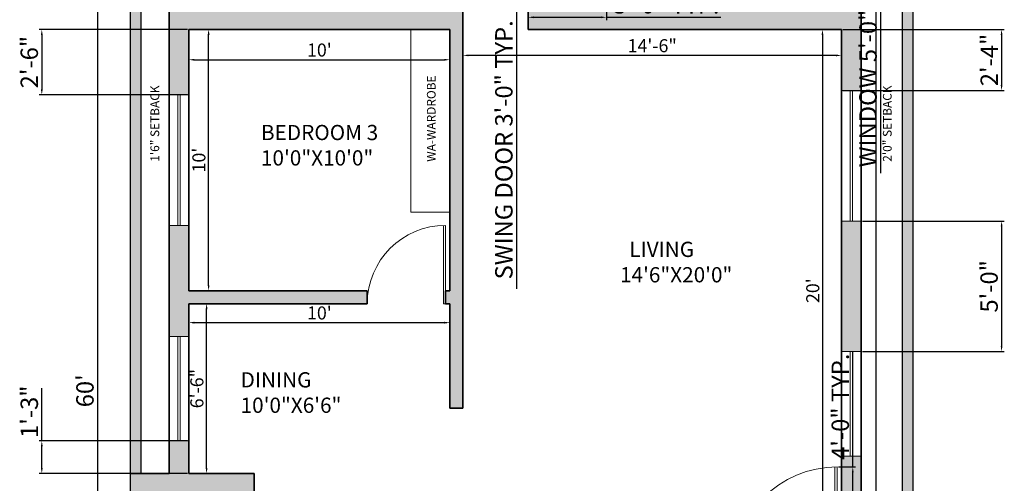
# Model space of a CAD drawing. Units: inches. Extents: x 2700 to 4052, y 1030 to 1872.
# Tile 7 of 8: x 3518 to 3971, y 1419 to 1632. Entities that reach past the tile are written whole.
import ezdxf

# ---------------------------------------------------------------- set-up
doc = ezdxf.new("R2010")
doc.units = ezdxf.units.IN
for name, color, linetype, lineweight in [('A-ANNO-DIMS', 2, 'Continuous', 13), ('A-ANNO-TEXT', 7, 'Continuous', 18), ('A-AREA-IDEN', 7, 'Continuous', 18), ('A-DOOR', 4, 'Continuous', 18), ('A-FLOR-CASE', 8, 'Continuous', 18), ('A-GLAZ', 4, 'Continuous', 18), ('A-WALL', 7, 'Continuous', 35), ('A-WALL-PATT', 7, 'Continuous', 13), ('C-PROP', 7, 'Continuous', 25)]:
    doc.layers.add(name, color=color, linetype=linetype, lineweight=lineweight)
doc.layers.add('C-SITE-PATT', color=252, linetype='Continuous', lineweight=13, true_color=0x939598)
doc.styles.get("Standard").update_dxf_attribs({"font": 'arial.ttf'})
doc.dimstyles.new('ISO-25', dxfattribs={"dimtxt": 8, "dimasz": 2.5, "dimexe": 1.25, "dimexo": 0.625, "dimtad": 1, "dimdec": 1, "dimlunit": 3, "dimtxsty": 'Standard', "dimcen": 2.5, "dimclrt": 1, "dimadec": 0, "dimazin": 0, "dimtfac": 1, "dimtdec": 1, "dimtmove": 0, "dimatfit": 3, "dimfxl": 1, "dimarcsym": 0})

# ---------------------------------------------------------------- blocks, each defined once
blk = doc.blocks.new('*D22')
at = {"layer": 'A-ANNO-DIMS', "color": 0, "lineweight": -2, "transparency": 16777216}
for p, q in [((3568.26, 1821.52), (3552.61, 1821.52)), ((3553.86, 1819.02), (3553.86, 1104.02)), ((3568.26, 1101.52), (3552.61, 1101.52))]:
    blk.add_line(p, q, dxfattribs=at)
at = {"layer": 'A-ANNO-DIMS', "color": 0, "transparency": 16777216}
for points in [[(3553.44, 1819.02), (3554.28, 1819.02), (3553.86, 1821.52)], [(3553.44, 1104.02), (3554.28, 1104.02), (3553.86, 1101.52)]]:
    blk.add_solid(points, dxfattribs=at)
at = {"layer": 'Defpoints', "color": 0, "transparency": 16777216}
for p in [(3568.88, 1821.52), (3553.86, 1101.52), (3568.88, 1101.52)]:
    blk.add_point(p, dxfattribs=at)
at = {"layer": 'A-ANNO-DIMS', "color": 0, "transparency": 16777216, "insert": (3549.15, 1461.52), "char_height": 8, "attachment_point": 5, "rotation": 90}
blk.add_mtext("60'", dxfattribs=at)
blk = doc.blocks.new('*D36')
at = {"layer": 'A-ANNO-DIMS', "color": 0, "lineweight": -2, "transparency": 16777216}
for p, q in [((3596.51, 1501.52), (3605.29, 1501.52)), ((3604.04, 1426.02), (3604.04, 1499.02)), ((3596.51, 1423.52), (3605.29, 1423.52))]:
    blk.add_line(p, q, dxfattribs=at)
at = {"layer": 'A-ANNO-DIMS', "color": 0, "transparency": 16777216}
for points in [[(3603.62, 1499.02), (3604.45, 1499.02), (3604.04, 1501.52)], [(3603.62, 1426.02), (3604.45, 1426.02), (3604.04, 1423.52)]]:
    blk.add_solid(points, dxfattribs=at)
at = {"layer": 'Defpoints', "color": 0, "transparency": 16777216}
for p in [(3595.88, 1501.52), (3604.04, 1501.52), (3595.88, 1423.52)]:
    blk.add_point(p, dxfattribs=at)
at = {"layer": 'A-ANNO-DIMS', "color": 0, "transparency": 16777216, "insert": (3600.35, 1462.52), "char_height": 6, "attachment_point": 5, "rotation": 90}
blk.add_mtext('6\'-6"', dxfattribs=at)
blk = doc.blocks.new('*D37')
at = {"layer": 'A-ANNO-DIMS', "color": 0, "lineweight": -2, "transparency": 16777216}
for p, q in [((3595.88, 1500.89), (3595.88, 1491.57)), ((3715.88, 1500.89), (3715.88, 1491.57)), ((3598.38, 1492.82), (3713.38, 1492.82))]:
    blk.add_line(p, q, dxfattribs=at)
at = {"layer": 'A-ANNO-DIMS', "color": 0, "transparency": 16777216}
for points in [[(3598.38, 1493.24), (3598.38, 1492.4), (3595.88, 1492.82)], [(3713.38, 1493.24), (3713.38, 1492.4), (3715.88, 1492.82)]]:
    blk.add_solid(points, dxfattribs=at)
at = {"layer": 'Defpoints', "color": 0, "transparency": 16777216}
for p in [(3595.88, 1501.52), (3715.88, 1501.52), (3715.88, 1492.82)]:
    blk.add_point(p, dxfattribs=at)
at = {"layer": 'A-ANNO-DIMS', "color": 0, "transparency": 16777216, "insert": (3655.88, 1496.51), "char_height": 6, "attachment_point": 5}
blk.add_mtext("10'", dxfattribs=at)
blk = doc.blocks.new('*D38')
at = {"layer": 'A-ANNO-DIMS', "color": 0, "lineweight": -2, "transparency": 16777216}
for p, q in [((3596.51, 1627.52), (3606.21, 1627.52)), ((3604.96, 1510.02), (3604.96, 1625.02)), ((3596.51, 1507.52), (3606.21, 1507.52))]:
    blk.add_line(p, q, dxfattribs=at)
at = {"layer": 'A-ANNO-DIMS', "color": 0, "transparency": 16777216}
for points in [[(3604.54, 1625.02), (3605.38, 1625.02), (3604.96, 1627.52)], [(3604.54, 1510.02), (3605.38, 1510.02), (3604.96, 1507.52)]]:
    blk.add_solid(points, dxfattribs=at)
at = {"layer": 'Defpoints', "color": 0, "transparency": 16777216}
for p in [(3595.88, 1627.52), (3604.96, 1627.52), (3595.88, 1507.52)]:
    blk.add_point(p, dxfattribs=at)
at = {"layer": 'A-ANNO-DIMS', "color": 0, "transparency": 16777216, "insert": (3601.27, 1567.52), "char_height": 6, "attachment_point": 5, "rotation": 90}
blk.add_mtext("10'", dxfattribs=at)
blk = doc.blocks.new('*D39')
at = {"layer": 'A-ANNO-DIMS', "color": 0, "lineweight": -2, "transparency": 16777216}
for p, q in [((3595.88, 1626.89), (3595.88, 1612.37)), ((3715.88, 1626.89), (3715.88, 1612.37)), ((3598.38, 1613.62), (3713.38, 1613.62))]:
    blk.add_line(p, q, dxfattribs=at)
at = {"layer": 'A-ANNO-DIMS', "color": 0, "transparency": 16777216}
for points in [[(3598.38, 1614.04), (3598.38, 1613.2), (3595.88, 1613.62)], [(3713.38, 1614.04), (3713.38, 1613.2), (3715.88, 1613.62)]]:
    blk.add_solid(points, dxfattribs=at)
at = {"layer": 'Defpoints', "color": 0, "transparency": 16777216}
for p in [(3595.88, 1627.52), (3715.88, 1627.52), (3715.88, 1613.62)]:
    blk.add_point(p, dxfattribs=at)
at = {"layer": 'A-ANNO-DIMS', "color": 0, "transparency": 16777216, "insert": (3655.88, 1617.31), "char_height": 6, "attachment_point": 5}
blk.add_mtext("10'", dxfattribs=at)
blk = doc.blocks.new('*D47')
at = {"layer": 'A-ANNO-DIMS', "color": 0, "lineweight": -2, "transparency": 16777216}
for p, q in [((3721.88, 1626.89), (3721.88, 1614.36)), ((3895.88, 1626.89), (3895.88, 1614.36)), ((3893.38, 1615.61), (3724.38, 1615.61))]:
    blk.add_line(p, q, dxfattribs=at)
at = {"layer": 'A-ANNO-DIMS', "color": 0, "transparency": 16777216}
for points in [[(3724.38, 1616.03), (3724.38, 1615.2), (3721.88, 1615.61)], [(3893.38, 1616.03), (3893.38, 1615.2), (3895.88, 1615.61)]]:
    blk.add_solid(points, dxfattribs=at)
at = {"layer": 'Defpoints', "color": 0, "transparency": 16777216}
for p in [(3721.88, 1627.52), (3895.88, 1627.52), (3721.88, 1615.61)]:
    blk.add_point(p, dxfattribs=at)
at = {"layer": 'A-ANNO-DIMS', "color": 0, "transparency": 16777216, "insert": (3808.88, 1619.3), "char_height": 6, "attachment_point": 5}
blk.add_mtext('14\'-6"', dxfattribs=at)
blk = doc.blocks.new('*D49')
at = {"layer": 'A-ANNO-DIMS', "color": 0, "lineweight": -2, "transparency": 16777216}
for p, q in [((3895.26, 1627.52), (3885.9, 1627.52)), ((3887.15, 1625.02), (3887.15, 1390.02)), ((3895.26, 1387.52), (3885.9, 1387.52))]:
    blk.add_line(p, q, dxfattribs=at)
at = {"layer": 'A-ANNO-DIMS', "color": 0, "transparency": 16777216}
for points in [[(3886.73, 1625.02), (3887.57, 1625.02), (3887.15, 1627.52)], [(3886.73, 1390.02), (3887.57, 1390.02), (3887.15, 1387.52)]]:
    blk.add_solid(points, dxfattribs=at)
at = {"layer": 'Defpoints', "color": 0, "transparency": 16777216}
for p in [(3895.88, 1627.52), (3887.15, 1387.52), (3895.88, 1387.52)]:
    blk.add_point(p, dxfattribs=at)
at = {"layer": 'A-ANNO-DIMS', "color": 0, "transparency": 16777216, "insert": (3883.46, 1507.52), "char_height": 6, "attachment_point": 5, "rotation": 90}
blk.add_mtext("20'", dxfattribs=at)
blk = doc.blocks.new('DOOR-SWING-48IN')
for p, q in [((-1, 48), (-1, 0)), ((0, 48), (0, 0)), ((0, 0), (-1, 0))]:
    blk.add_line(p, q)
blk.add_arc((0, 0), 48, 90, 180)
blk = doc.blocks.new('DOOR-SWING-36IN')
for p, q in [((-1, 36), (-1, 0)), ((0, 36), (0, 0)), ((0, 0), (-1, 0))]:
    blk.add_line(p, q)
blk.add_arc((0, 0), 36, 90, 180)
blk = doc.blocks.new('WINDOW-48IN')
for p, q in [((-24, -4.5), (-24, 4.5)), ((-24, 0.5), (24, 0.5)), ((24, -4.5), (24, 4.5)), ((-24, -0.5), (24, -0.5))]:
    blk.add_line(p, q)
blk = doc.blocks.new('WINDOW-60IN')
for p, q in [((4.5, 30), (-4.5, 30)), ((-0.5, 30), (-0.5, -30)), ((0.5, 30), (0.5, -30)), ((4.5, -30), (-4.5, -30))]:
    blk.add_line(p, q)
blk = doc.blocks.new('*D66')
at = {"layer": 'A-ANNO-DIMS', "color": 0, "lineweight": -2, "transparency": 16777216}
for p, q in [((3905.51, 1726.52), (3915.13, 1726.52)), ((3913.88, 1724.02), (3913.88, 1669.02)), ((3905.51, 1666.52), (3915.13, 1666.52)), ((3913.88, 1666.52), (3913.88, 1561.53))]:
    blk.add_line(p, q, dxfattribs=at)
at = {"layer": 'A-ANNO-DIMS', "color": 0, "transparency": 16777216}
for points in [[(3913.47, 1724.02), (3914.3, 1724.02), (3913.88, 1726.52)], [(3913.47, 1669.02), (3914.3, 1669.02), (3913.88, 1666.52)]]:
    blk.add_solid(points, dxfattribs=at)
at = {"layer": 'Defpoints', "color": 0, "transparency": 16777216}
for p in [(3904.88, 1726.52), (3904.88, 1666.52), (3913.88, 1666.52)]:
    blk.add_point(p, dxfattribs=at)
at = {"layer": 'A-ANNO-DIMS', "color": 1, "transparency": 16777216, "insert": (3909.12, 1612.78), "char_height": 8, "attachment_point": 5, "rotation": 90}
blk.add_mtext('WINDOW 5\'-0" TYP.', dxfattribs=at)
blk = doc.blocks.new('*D70')
at = {"layer": 'A-ANNO-DIMS', "color": 0, "lineweight": -2, "transparency": 16777216}
for p, q in [((3751.26, 1674.52), (3745.23, 1674.52)), ((3746.48, 1672.02), (3746.48, 1641.02)), ((3751.26, 1638.52), (3745.23, 1638.52)), ((3746.48, 1638.52), (3746.48, 1508.43))]:
    blk.add_line(p, q, dxfattribs=at)
at = {"layer": 'A-ANNO-DIMS', "color": 0, "transparency": 16777216}
for points in [[(3746.07, 1672.02), (3746.9, 1672.02), (3746.48, 1674.52)], [(3746.07, 1641.02), (3746.9, 1641.02), (3746.48, 1638.52)]]:
    blk.add_solid(points, dxfattribs=at)
at = {"layer": 'Defpoints', "color": 0, "transparency": 16777216}
for p in [(3751.88, 1674.52), (3746.48, 1638.52), (3751.88, 1638.52)]:
    blk.add_point(p, dxfattribs=at)
at = {"layer": 'A-ANNO-DIMS', "color": 1, "transparency": 16777216, "insert": (3741.72, 1572.22), "char_height": 8, "attachment_point": 5, "rotation": 90}
blk.add_mtext('SWING DOOR 3\'-0" TYP.', dxfattribs=at)
blk = doc.blocks.new('*D71')
at = {"layer": 'A-ANNO-DIMS', "color": 0, "lineweight": -2, "transparency": 16777216}
for p, q in [((3751.88, 1637.89), (3751.88, 1631.87)), ((3787.88, 1637.89), (3787.88, 1631.87)), ((3754.38, 1633.12), (3785.38, 1633.12)), ((3787.88, 1633.12), (3840.39, 1633.12))]:
    blk.add_line(p, q, dxfattribs=at)
at = {"layer": 'A-ANNO-DIMS', "color": 0, "transparency": 16777216}
for points in [[(3754.38, 1633.53), (3754.38, 1632.7), (3751.88, 1633.12)], [(3785.38, 1633.53), (3785.38, 1632.7), (3787.88, 1633.12)]]:
    blk.add_solid(points, dxfattribs=at)
at = {"layer": 'Defpoints', "color": 0, "transparency": 16777216}
for p in [(3751.88, 1638.52), (3787.88, 1638.52), (3787.88, 1633.12)]:
    blk.add_point(p, dxfattribs=at)
at = {"layer": 'A-ANNO-DIMS', "color": 1, "transparency": 16777216, "insert": (3815.39, 1637.83), "char_height": 8, "attachment_point": 5}
blk.add_mtext('3\'-0" TYP.', dxfattribs=at)
blk = doc.blocks.new('*D75')
at = {"layer": 'A-ANNO-DIMS', "color": 0, "lineweight": -2, "transparency": 16777216}
for p, q in [((3901.08, 1426.52), (3901.08, 1479.35)), ((3894.51, 1426.52), (3902.33, 1426.52)), ((3901.08, 1381.02), (3901.08, 1424.02)), ((3894.51, 1378.52), (3902.33, 1378.52))]:
    blk.add_line(p, q, dxfattribs=at)
at = {"layer": 'A-ANNO-DIMS', "color": 0, "transparency": 16777216}
for points in [[(3900.67, 1424.02), (3901.5, 1424.02), (3901.08, 1426.52)], [(3900.67, 1381.02), (3901.5, 1381.02), (3901.08, 1378.52)]]:
    blk.add_solid(points, dxfattribs=at)
at = {"layer": 'Defpoints', "color": 0, "transparency": 16777216}
for p in [(3893.88, 1426.52), (3901.08, 1426.52), (3893.88, 1378.52)]:
    blk.add_point(p, dxfattribs=at)
at = {"layer": 'A-ANNO-DIMS', "color": 1, "transparency": 16777216, "insert": (3896.37, 1454.19), "char_height": 8, "attachment_point": 5, "rotation": 90}
blk.add_mtext('4\'-0" TYP.', dxfattribs=at)
blk = doc.blocks.new('*D104')
at = {"layer": 'A-ANNO-DIMS', "color": 0, "lineweight": -2, "transparency": 16777216}
for p, q in [((3911.88, 1102.14), (3911.88, 1863.37)), ((3914.38, 1862.12), (3926.38, 1862.12)), ((3928.88, 1102.14), (3928.88, 1863.37)), ((3928.88, 1862.12), (3953.15, 1862.12))]:
    blk.add_line(p, q, dxfattribs=at)
at = {"layer": 'A-ANNO-DIMS', "color": 0, "transparency": 16777216}
for points in [[(3914.38, 1862.53), (3914.38, 1861.7), (3911.88, 1862.12)], [(3926.38, 1862.53), (3926.38, 1861.7), (3928.88, 1862.12)]]:
    blk.add_solid(points, dxfattribs=at)
at = {"layer": 'Defpoints', "color": 0, "transparency": 16777216}
for p in [(3928.88, 1862.12), (3911.88, 1101.52), (3928.88, 1101.52)]:
    blk.add_point(p, dxfattribs=at)
at = {"layer": 'A-ANNO-DIMS', "color": 1, "transparency": 16777216, "insert": (3942.26, 1866.83), "char_height": 8, "attachment_point": 5}
blk.add_mtext('1\'-5"', dxfattribs=at)
blk = doc.blocks.new('*D107')
at = {"layer": 'A-ANNO-DIMS', "color": 0, "lineweight": -2, "transparency": 16777216}
for p, q in [((3595.26, 1627.52), (3527.03, 1627.52)), ((3528.28, 1625.02), (3528.28, 1600.02)), ((3595.26, 1597.52), (3527.03, 1597.52))]:
    blk.add_line(p, q, dxfattribs=at)
at = {"layer": 'A-ANNO-DIMS', "color": 0, "transparency": 16777216}
for points in [[(3527.87, 1625.02), (3528.7, 1625.02), (3528.28, 1627.52)], [(3527.87, 1600.02), (3528.7, 1600.02), (3528.28, 1597.52)]]:
    blk.add_solid(points, dxfattribs=at)
at = {"layer": 'Defpoints', "color": 0, "transparency": 16777216}
for p in [(3595.88, 1627.52), (3528.28, 1597.52), (3595.88, 1597.52)]:
    blk.add_point(p, dxfattribs=at)
at = {"layer": 'A-ANNO-DIMS', "color": 1, "transparency": 16777216, "insert": (3523.57, 1612.52), "char_height": 8, "attachment_point": 5, "rotation": 90}
blk.add_mtext('2\'-6"', dxfattribs=at)
blk = doc.blocks.new('*D108')
at = {"layer": 'A-ANNO-DIMS', "color": 0, "lineweight": -2, "transparency": 16777216}
for p, q in [((3528.28, 1438.52), (3528.28, 1462.78)), ((3595.26, 1438.52), (3527.03, 1438.52)), ((3528.28, 1426.02), (3528.28, 1436.02)), ((3595.26, 1423.52), (3527.03, 1423.52))]:
    blk.add_line(p, q, dxfattribs=at)
at = {"layer": 'A-ANNO-DIMS', "color": 0, "transparency": 16777216}
for points in [[(3527.87, 1436.02), (3528.7, 1436.02), (3528.28, 1438.52)], [(3527.87, 1426.02), (3528.7, 1426.02), (3528.28, 1423.52)]]:
    blk.add_solid(points, dxfattribs=at)
at = {"layer": 'Defpoints', "color": 0, "transparency": 16777216}
for p in [(3528.28, 1438.52), (3595.88, 1438.52), (3595.88, 1423.52)]:
    blk.add_point(p, dxfattribs=at)
at = {"layer": 'A-ANNO-DIMS', "color": 1, "transparency": 16777216, "insert": (3523.57, 1451.9), "char_height": 8, "attachment_point": 5, "rotation": 90}
blk.add_mtext('1\'-3"', dxfattribs=at)
blk = doc.blocks.new('*D110')
at = {"layer": 'A-ANNO-DIMS', "color": 0, "lineweight": -2, "transparency": 16777216}
for p, q in [((3896.51, 1627.52), (3970.73, 1627.52)), ((3969.48, 1625.02), (3969.48, 1602.02)), ((3896.51, 1599.52), (3970.73, 1599.52))]:
    blk.add_line(p, q, dxfattribs=at)
at = {"layer": 'A-ANNO-DIMS', "color": 0, "transparency": 16777216}
for points in [[(3969.07, 1625.02), (3969.9, 1625.02), (3969.48, 1627.52)], [(3969.07, 1602.02), (3969.9, 1602.02), (3969.48, 1599.52)]]:
    blk.add_solid(points, dxfattribs=at)
at = {"layer": 'Defpoints', "color": 0, "transparency": 16777216}
for p in [(3895.88, 1627.52), (3895.88, 1599.52), (3969.48, 1599.52)]:
    blk.add_point(p, dxfattribs=at)
at = {"layer": 'A-ANNO-DIMS', "color": 1, "transparency": 16777216, "insert": (3964.84, 1613.52), "char_height": 8, "attachment_point": 5, "rotation": 90}
blk.add_mtext('2\'-4"', dxfattribs=at)
blk = doc.blocks.new('*D115')
at = {"layer": 'A-ANNO-DIMS', "color": 0, "lineweight": -2, "transparency": 16777216}
for p, q in [((3905.51, 1539.52), (3970.73, 1539.52)), ((3969.48, 1537.02), (3969.48, 1482.02)), ((3905.51, 1479.52), (3970.73, 1479.52))]:
    blk.add_line(p, q, dxfattribs=at)
at = {"layer": 'A-ANNO-DIMS', "color": 0, "transparency": 16777216}
for points in [[(3969.07, 1537.02), (3969.9, 1537.02), (3969.48, 1539.52)], [(3969.07, 1482.02), (3969.9, 1482.02), (3969.48, 1479.52)]]:
    blk.add_solid(points, dxfattribs=at)
at = {"layer": 'Defpoints', "color": 0, "transparency": 16777216}
for p in [(3904.88, 1539.52), (3904.88, 1479.52), (3969.48, 1479.52)]:
    blk.add_point(p, dxfattribs=at)
at = {"layer": 'A-ANNO-DIMS', "color": 1, "transparency": 16777216, "insert": (3964.77, 1509.52), "char_height": 8, "attachment_point": 5, "rotation": 90}
blk.add_mtext('5\'-0"', dxfattribs=at)

msp = doc.modelspace()

# ---------------------------------------------------------------- hatches: boundary and pattern name
at = {"layer": 'A-WALL-PATT'}
h = msp.add_hatch(color=256, dxfattribs=at)
h.dxf.hatch_style = 1
h.paths.add_polyline_path([(3904.88, 1539.52), (3895.88, 1539.52), (3895.88, 1479.52), (3904.88, 1479.52)])
h.paths.add_polyline_path([(3904.88, 1666.52), (3895.88, 1666.52), (3895.88, 1636.52), (3760.88, 1636.52), (3760.88, 1638.52), (3751.88, 1638.52), (3751.88, 1627.52), (3868.81, 1627.52, -0.035851), (3872.34, 1627.52), (3895.88, 1627.52), (3895.88, 1599.52), (3904.88, 1599.52)])
h.paths.add_polyline_path([(3595.88, 1537.52), (3586.88, 1537.52), (3586.88, 1486.52), (3595.88, 1486.52), (3595.88, 1501.52), (3677.88, 1501.52), (3677.88, 1507.52), (3595.88, 1507.52)], flags=17)
h.paths.add_polyline_path([(3595.88, 1438.52), (3586.88, 1438.52), (3586.88, 1423.52), (3568.88, 1423.52), (3568.88, 1414.52), (3616.88, 1414.52), (3616.88, 1412.52), (3625.88, 1412.52), (3625.88, 1423.52), (3595.88, 1423.52)])
h.paths.add_polyline_path([(3721.88, 1636.52), (3706.88, 1636.52), (3706.88, 1638.52), (3697.88, 1638.52), (3697.88, 1636.52), (3595.88, 1636.52), (3595.88, 1685.52), (3586.88, 1685.52), (3586.88, 1597.52), (3595.88, 1597.52), (3595.88, 1627.52), (3715.88, 1627.52), (3715.88, 1507.52), (3713.88, 1507.52), (3713.88, 1501.52), (3715.88, 1501.52), (3715.88, 1453.52), (3721.88, 1453.52)])
h.paths.add_polyline_path([(3724.88, 1756.52), (3863.88, 1756.52), (3863.88, 1762.52), (3814.88, 1762.52), (3814.88, 1812.52), (3895.88, 1812.52), (3895.88, 1799.52), (3904.88, 1799.52), (3904.88, 1821.52), (3796.88, 1821.52), (3796.88, 1812.52), (3808.88, 1812.52), (3808.88, 1762.52), (3724.88, 1762.52), (3724.88, 1764.52), (3715.88, 1764.52), (3715.88, 1686.52), (3697.88, 1686.52), (3697.88, 1674.52), (3706.88, 1674.52), (3706.88, 1677.52), (3751.88, 1677.52), (3751.88, 1674.52), (3760.88, 1674.52), (3760.88, 1686.52), (3724.88, 1686.52)])
h.paths.add_polyline_path([(3904.88, 1775.52), (3895.88, 1775.52), (3895.88, 1762.52), (3893.88, 1762.52), (3893.88, 1756.52), (3895.88, 1756.52), (3895.88, 1726.52), (3904.88, 1726.52)], flags=17)
h.paths.add_polyline_path([(3772.88, 1821.52), (3586.88, 1821.52), (3586.88, 1745.52), (3595.88, 1745.52), (3595.88, 1812.52), (3715.88, 1812.52), (3715.88, 1794.52), (3724.88, 1794.52), (3724.88, 1812.52), (3772.88, 1812.52)])
h = msp.add_hatch(color=256, dxfattribs=at)
h.dxf.hatch_style = 1
h.paths.add_polyline_path([(3651.88, 1264.52), (3625.88, 1264.52), (3625.88, 1310.49), (3616.88, 1310.49), (3616.88, 1304.37), (3616.88, 1264.52), (3568.88, 1264.52), (3568.88, 1168.52), (3709.88, 1168.52), (3709.88, 1177.52), (3577.88, 1177.52), (3577.88, 1255.52), (3651.88, 1255.52)])
h.paths.add_polyline_path([(3740.88, 1264.52), (3734.88, 1264.52), (3734.88, 1324.52), (3782.88, 1324.52), (3782.88, 1264.52), (3776.88, 1264.52), (3776.88, 1255.52), (3791.88, 1255.52), (3791.88, 1378.52), (3794.88, 1378.52), (3794.88, 1387.52), (3776.88, 1387.52), (3776.88, 1381.52), (3782.88, 1381.52), (3782.88, 1333.52), (3734.88, 1333.52), (3734.88, 1381.52), (3740.88, 1381.52), (3740.88, 1387.52), (3725.88, 1387.52), (3725.88, 1264.52), (3699.88, 1264.52), (3699.88, 1255.52), (3740.88, 1255.52)])
h.paths.add_polyline_path([(3625.88, 1382.52), (3616.88, 1382.52), (3616.88, 1358.49), (3625.88, 1358.49)])
h.paths.add_polyline_path([(3845.88, 1387.52), (3842.88, 1387.52), (3842.88, 1378.52), (3845.88, 1378.52)])
h.paths.add_polyline_path([(3904.88, 1431.52), (3895.88, 1431.52), (3895.88, 1387.52), (3893.88, 1387.52), (3893.88, 1378.52), (3895.88, 1378.52), (3895.88, 1300.52), (3904.88, 1300.52)])
h.paths.add_polyline_path([(3584.49, 1565.14), (3584.49, 1604.05), (3576.25, 1604.05), (3576.25, 1565.14)], flags=9)
h.paths.add_polyline_path([(3711.56, 1565.68), (3711.56, 1611.46), (3703.32, 1611.46), (3703.32, 1565.68)], flags=9)
h.paths.add_polyline_path([(3737.75, 1697.89), (3737.75, 1743.66), (3729.51, 1743.66), (3729.51, 1697.89)], flags=9)
h.paths.add_polyline_path([(3633.29, 1800.61), (3679.06, 1800.61), (3679.06, 1808.85), (3633.29, 1808.85)], flags=9)
h.paths.add_polyline_path([(3569.7, 1361.72), (3618.67, 1361.72), (3618.67, 1388.34), (3569.7, 1388.34)], flags=9)
h.paths.add_polyline_path([(3658.81, 1318.27), (3708.12, 1318.27), (3708.12, 1344.89), (3658.81, 1344.89)], flags=9)
h.paths.add_polyline_path([(3791.11, 1507.34), (3845.25, 1507.34), (3845.25, 1533.96), (3791.11, 1533.96)], flags=9)
h.paths.add_polyline_path([(3744.61, 1774.23), (3794.63, 1774.23), (3794.63, 1800.84), (3744.61, 1800.84)], flags=9)
h.paths.add_polyline_path([(3831.1, 1774.23), (3881.17, 1774.23), (3881.17, 1800.84), (3831.1, 1800.84)], flags=9)
h.paths.add_polyline_path([(3791.11, 1664.37), (3855.09, 1664.37), (3855.09, 1690.98), (3791.11, 1690.98)], flags=9)
h.paths.add_polyline_path([(3626.06, 1747.79), (3690.04, 1747.79), (3690.04, 1774.41), (3626.06, 1774.41)], flags=9)
h.paths.add_polyline_path([(3626.06, 1590.97), (3690.04, 1590.97), (3690.04, 1617.58), (3626.06, 1617.58)], flags=9)
h.paths.add_polyline_path([(3616.71, 1447.4), (3665.68, 1447.4), (3665.68, 1474.01), (3616.71, 1474.01)], flags=9)
at = {"layer": 'C-SITE-PATT'}
h = msp.add_hatch(color=256, dxfattribs=at)
h.dxf.hatch_style = 1
h.paths.add_polyline_path([(3573.88, 1821.52), (3568.88, 1821.52), (3568.88, 1423.52), (3573.88, 1423.52)])
h.paths.add_polyline_path([(3791.88, 1108.52), (3573.88, 1108.52), (3573.88, 1168.52), (3568.88, 1168.52), (3568.88, 1101.52), (3791.88, 1101.52)])
h.paths.add_polyline_path([(3928.88, 1821.52), (3923.88, 1821.52), (3923.88, 1108.52), (3911.88, 1108.52), (3911.88, 1101.52), (3928.88, 1101.52)])

# ---------------------------------------------------------------- linework, layer by layer
at = {"layer": 'A-FLOR-CASE'}
for p in [(3697.88, 1627.52), (3715.88, 1543.52)]:
    msp.add_line(p, (3697.88, 1543.52), dxfattribs=at)
at = {"layer": 'A-WALL'}
for p, q in [((3586.88, 1821.52), (3586.88, 1423.52)), ((3904.88, 1300.52), (3904.88, 1821.52)), ((3751.88, 1638.52), (3751.88, 1627.52)), ((3721.88, 1636.52), (3721.88, 1453.52)), ((3715.88, 1627.52), (3595.88, 1627.52)), ((3595.88, 1627.52), (3595.88, 1507.52)), ((3715.88, 1627.52), (3715.88, 1507.52)), ((3895.88, 1627.52), (3751.88, 1627.52)), ((3895.88, 1387.52), (3895.88, 1627.52)), ((3677.88, 1507.52), (3595.88, 1507.52)), ((3677.88, 1507.52), (3677.88, 1501.52)), ((3715.88, 1507.52), (3713.88, 1507.52)), ((3713.88, 1507.52), (3713.88, 1501.52)), ((3677.88, 1501.52), (3595.88, 1501.52)), ((3595.88, 1501.52), (3595.88, 1423.52)), ((3715.88, 1501.52), (3713.88, 1501.52)), ((3715.88, 1501.52), (3715.88, 1453.52)), ((3721.88, 1453.52), (3715.88, 1453.52)), ((3586.88, 1423.52), (3568.88, 1423.52)), ((3625.88, 1423.52), (3595.88, 1423.52)), ((3625.88, 1412.52), (3625.88, 1423.52))]:
    msp.add_line(p, q, dxfattribs=at)
at = {"layer": 'C-PROP'}
for p, q in [((3573.88, 1821.52), (3573.88, 1423.52)), ((3923.88, 1108.52), (3923.88, 1821.52))]:
    msp.add_line(p, q, dxfattribs=at)
msp.add_lwpolyline([(3911.88, 1101.52), (3928.88, 1101.52), (3928.88, 1821.52), (3568.88, 1821.52), (3568.88, 1101.52), (3791.88, 1101.52)], dxfattribs=at)

# ---------------------------------------------------------------- block references
at = {"layer": 'A-DOOR'}
for name, p in [('DOOR-SWING-36IN', (3713.88, 1501.52)), ('DOOR-SWING-48IN', (3893.88, 1378.52))]:
    msp.add_blockref(name, p, dxfattribs=at)
at = {"layer": 'A-GLAZ'}
for p in [(3900.38, 1569.52), (3591.38, 1567.52)]:
    msp.add_blockref('WINDOW-60IN', p, dxfattribs=at)
for p, rotation in [((3591.38, 1462.52), 90.00000000000595), ((3900.38, 1455.52), 90.00000000000384)]:
    msp.add_blockref('WINDOW-48IN', p, dxfattribs=dict(at, rotation=rotation))

# ---------------------------------------------------------------- texts
at = {"layer": 'A-ANNO-TEXT', "char_height": 4, "attachment_point": 1, "rotation": 90}
for s, width, insert in [('WA-WARDROBE', 29.5334, (3705.31, 1566.75)), ('1\'6" SETBACK', 45.8842, (3578.24, 1566.75)), ('2\'0" SETBACK', 41.5432, (3914.94, 1566.75))]:
    msp.add_mtext_dynamic_manual_height_columns(s, width=width, gutter_width=12.5, heights=[0], dxfattribs=dict(at, insert=insert))
at = {"layer": 'A-AREA-IDEN', "char_height": 7, "attachment_point": 1}
for s, insert in [('{\\fTimes New Roman|b0|i0|c0|p18;BEDROOM 3\\P10\'0"X10\'0"}', (3629.02, 1583.69)), ('{\\fTimes New Roman|b0|i0|c0|p18;  LIVING\\P14\'6"X20\'0"}', (3794.08, 1530)), ('{\\fTimes New Roman|b0|i0|c0|p18;DINING\\P10\'0"X6\'6"}', (3619.67, 1470.05))]:
    msp.add_mtext_dynamic_manual_height_columns(s, width=61.0557, gutter_width=12.5, heights=[0], dxfattribs=dict(at, insert=insert))

# ---------------------------------------------------------------- dimensions: what is measured, and where the dimension line sits
at = {"layer": 'A-ANNO-DIMS'}
for base, p1, p2, override, picture, middle in [((3928.88, 1862.12), (3911.88, 1101.52), (3928.88, 1101.52), {"dimdec": 1, "dimlfac": 1, "dimrnd": 0, "dimzin": 1, "dimdsep": 46, "dimlunit": 4, "dimfrac": 2}, '*D104', (3942.26, 1866.83)), ((3715.88, 1613.62), (3595.88, 1627.52), (3715.88, 1627.52), {"dimtxt": 6, "dimclrd": 0, "dimclre": 0, "dimclrt": 0}, '*D39', (3655.88, 1617.31)), ((3721.88, 1615.61), (3895.88, 1627.52), (3721.88, 1627.52), {"dimtxt": 6, "dimclrd": 0, "dimclre": 0, "dimclrt": 0}, '*D47', (3808.88, 1619.3)), ((3715.88, 1492.82), (3595.88, 1501.52), (3715.88, 1501.52), {"dimtxt": 6, "dimclrd": 0, "dimclre": 0, "dimclrt": 0}, '*D37', (3655.88, 1496.51))]:
    dim = msp.add_linear_dim(base=base, p1=p1, p2=p2, dimstyle='ISO-25', override=override, dxfattribs=at)
    dim.commit()
    dim.dimension.update_dxf_attribs({"geometry": picture, "text_midpoint": middle})
for base, p1, p2, angle, override, picture, middle in [((3553.86, 1101.52), (3568.88, 1821.52), (3568.88, 1101.52), 90, {"dimclrd": 0, "dimclre": 0, "dimclrt": 0}, '*D22', (3549.15, 1461.52)), ((3528.28, 1597.52), (3595.88, 1627.52), (3595.88, 1597.52), 90, {"dimdec": 1, "dimlfac": 1, "dimrnd": 0, "dimzin": 1, "dimdsep": 46, "dimlunit": 4, "dimfrac": 2}, '*D107', (3523.57, 1612.52)), ((3604.96, 1627.52), (3595.88, 1507.52), (3595.88, 1627.52), 270, {"dimtxt": 6, "dimclrd": 0, "dimclre": 0, "dimclrt": 0}, '*D38', (3601.27, 1567.52)), ((3887.15, 1387.52), (3895.88, 1627.52), (3895.88, 1387.52), 90, {"dimtxt": 6, "dimclrd": 0, "dimclre": 0, "dimclrt": 0}, '*D49', (3883.46, 1507.52)), ((3969.48, 1599.52), (3895.88, 1627.52), (3895.88, 1599.52), 90, {"dimdec": 1, "dimlfac": 1, "dimrnd": 0, "dimzin": 1, "dimdsep": 46, "dimlunit": 4, "dimfrac": 2}, '*D110', (3964.84, 1613.52)), ((3969.48, 1479.52), (3904.88, 1539.52), (3904.88, 1479.52), 90, {"dimdec": 1, "dimlfac": 1, "dimrnd": 0, "dimzin": 1, "dimdsep": 46, "dimlunit": 4, "dimfrac": 2}, '*D115', (3964.77, 1509.52)), ((3604.04, 1501.52), (3595.88, 1423.52), (3595.88, 1501.52), 270, {"dimtxt": 6, "dimclrd": 0, "dimclre": 0, "dimclrt": 0}, '*D36', (3600.35, 1462.52)), ((3528.28, 1438.52), (3595.88, 1423.52), (3595.88, 1438.52), 90, {"dimdec": 1, "dimlfac": 1, "dimrnd": 0, "dimzin": 1, "dimdsep": 46, "dimlunit": 4, "dimfrac": 2}, '*D108', (3523.57, 1451.9))]:
    dim = msp.add_linear_dim(base=base, p1=p1, p2=p2, angle=angle, dimstyle='ISO-25', override=override, dxfattribs=at)
    dim.commit()
    dim.dimension.update_dxf_attribs({"geometry": picture, "text_midpoint": middle})
for base, p1, p2, angle, text, picture, middle in [((3913.88, 1666.52), (3904.88, 1726.52), (3904.88, 1666.52), 270, 'WINDOW <> TYP.', '*D66', (3909.12, 1612.78)), ((3746.48, 1638.52), (3751.88, 1674.52), (3751.88, 1638.52), 270, 'SWING DOOR <> TYP.', '*D70', (3741.72, 1572.22)), ((3787.88, 1633.12), (3751.88, 1638.52), (3787.88, 1638.52), 0, '<> TYP.', '*D71', (3815.39, 1637.83)), ((3901.08, 1426.52), (3893.88, 1378.52), (3893.88, 1426.52), 90, '<> TYP.', '*D75', (3896.37, 1454.19))]:
    dim = msp.add_linear_dim(base=base, p1=p1, p2=p2, angle=angle, text=text, dimstyle='ISO-25', override={"dimdec": 1, "dimlfac": 1, "dimrnd": 0, "dimzin": 1, "dimdsep": 46, "dimlunit": 4, "dimfrac": 2}, dxfattribs=at)
    dim.commit()
    dim.dimension.update_dxf_attribs({"geometry": picture, "text_midpoint": middle})

doc.saveas('drawing.dxf')
